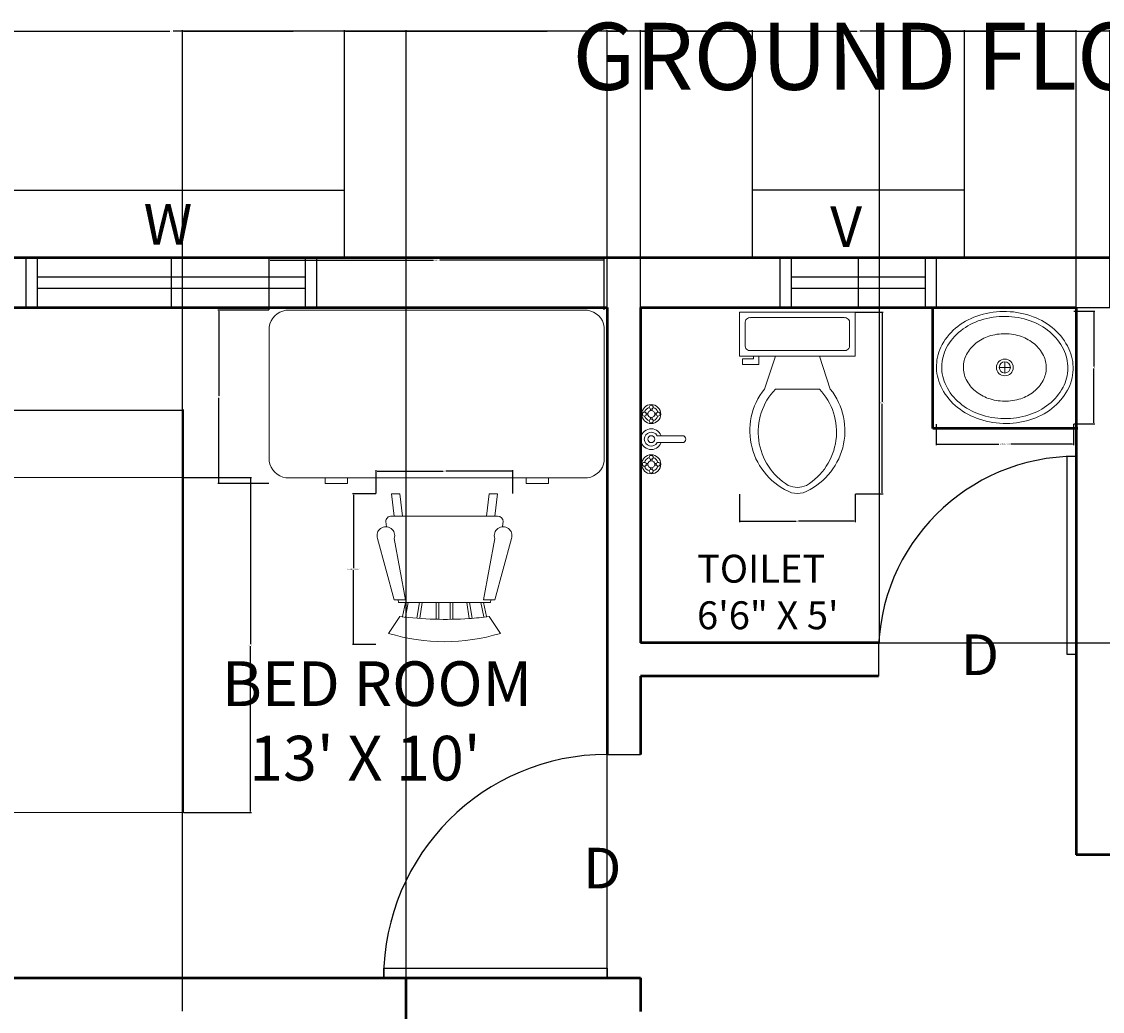
# Model space of a CAD drawing. Units: inches. Extents: x -73 to 1162, y -188 to 590.
# Tile 3 of 9: x 28 to 222, y 17 to 194. Entities that reach past the tile are written whole.
import ezdxf

# ---------------------------------------------------------------- set-up
doc = ezdxf.new("R2010")
doc.units = ezdxf.units.IN
doc.header["$MEASUREMENT"] = 0
for name, color, linetype, lineweight in [('A-ANNO-DIMS', 2, 'Continuous', 18), ('A-ANNO-TEXT', 7, 'Continuous', 25), ('A-AREA-IDEN', 2, 'Continuous', 25), ('A-DOOR', 3, 'Continuous', 25), ('A-FLOR-FIXT', 8, 'Continuous', 18), ('A-FURN', 8, 'Continuous', 18), ('A-GLAZ', 4, 'Continuous', 25), ('A-WALL', 7, 'Continuous', 50)]:
    doc.layers.add(name, color=color, linetype=linetype, lineweight=lineweight)
doc.styles.get("Standard").update_dxf_attribs({"font": 'arial.ttf'})
doc.dimstyles.get("Standard").update_dxf_attribs({"dimtxt": 0.18, "dimasz": 0.18, "dimexe": 0.18, "dimexo": 0.0625, "dimgap": 0.09, "dimtad": 0, "dimtih": 1, "dimtoh": 1, "dimdec": 1, "dimzin": 0, "dimdsep": 46, "dimlunit": 4, "dimtxsty": 'Standard', "dimcen": 0.09, "dimadec": 0, "dimazin": 0, "dimtfac": 1, "dimtdec": 1, "dimtofl": 0, "dimtmove": 0, "dimatfit": 3, "dimfxl": 1, "dimtolj": 1, "dimtzin": 0, "dimarcsym": 0})

# ---------------------------------------------------------------- blocks, each defined once
blk = doc.blocks.new('*U2')
for p, q in [((0, 0), (0, -6)), ((40, 0), (40, -6))]:
    blk.add_line(p, q)
blk.add_lwpolyline([(0, 0), (0, 40), (1.75, 40), (1.75, 0)], close=True)
blk.add_arc((0, 0), 40, 0, 90)
blk = doc.blocks.new('*U5')
for p, q in [((0, 0), (0, -100)), ((-900, 0), (-900, -100))]:
    blk.add_line(p, q)
blk.add_lwpolyline([(0, 0), (0, 900), (-43.75, 900), (-43.75, 0)], close=True)
blk.add_arc((0, 0), 900, 90, 180)
blk = doc.blocks.new('Bed - Queen')
for p, q in [((0, -80.00003), (0, 0)), ((0, 0), (59.99999, 0)), ((59.99999, 0), (59.99999, -80.00003)), ((7.99999, -1.2), (28.79998, -1.2)), ((7.99999, -14.4), (7.99999, -1.2)), ((28.79998, -1.2), (28.79998, -14.4)), ((31.19999, -1.2), (51.99999, -1.2)), ((31.19999, -14.4), (31.19999, -1.2)), ((51.99999, -1.2), (51.99999, -16.4)), ((0, -14.4), (44.8, -14.4)), ((59.99999, -29.6), (44.8, -14.4)), ((44.8, -14.4), (44.8, -29.6)), ((44.8, -16.8), (0, -16.8)), ((51.99999, -16.4), (46.79936, -16.4)), ((44.8, -29.6), (59.99999, -29.6)), ((59.99999, -80.00003), (0, -80.00003))]:
    blk.add_line(p, q)
blk = doc.blocks.new('Desk - 30 x 60 in.')
for p, q in [((-26.999995, 0), (26.999995, 0)), ((-29.999995, -27), (-29.999995, -3)), ((29.999995, -3), (29.999995, -27)), ((26.999995, -30), (-26.999995, -30)), ((-20.000005, -30), (-20.000005, -31)), ((-16.000005, -31), (-16.000005, -30)), ((15.999995, -31), (15.999995, -30)), ((19.999995, -30), (19.999995, -31)), ((-20.000005, -31), (-16.000005, -31)), ((19.999995, -31), (15.999995, -31))]:
    blk.add_line(p, q)
for centre, start, end in [((-26.499995, -3.5), 98.1301, 171.8699), ((26.499995, -3.5), 8.130102, 81.8699), ((-26.499995, -26.5), 188.1301, 261.8699), ((26.499995, -26.5), 278.1301, 351.8699)]:
    blk.add_arc(centre, 3.535534, start, end)
blk = doc.blocks.new('Chair - Rocking')
for p, q in [((-8, -4.5), (-10, -1.5)), ((8, -4.5), (10, -1.5)), ((-7.5, -4.5), (-7, -7)), ((-6.5, -7), (-7.02225, -4.43)), ((-4.5, -7), (-4.96674, -4.19951)), ((-4, -7), (-4.40532, -4.16272)), ((-1.5, -4.05012), (-1.5, -7)), ((-1, -7), (-1, -4.05012)), ((1, -7), (1, -4.04655)), ((1.5, -4.05012), (1.5, -7)), ((4, -7), (4.40187, -4.18694)), ((4.5, -7), (4.96761, -4.19437)), ((6.5, -7), (7, -4.4057)), ((7.5, -4.5), (7, -7)), ((-9, -7.5), (-12, -18.49999)), ((-7, -7.5), (-9, -7.5)), ((-9, -18.49999), (-7, -7.5)), ((-8.23428, -6.99939), (-8.3093, -7.47958)), ((-8.23041, -7), (8.23915, -7)), ((7, -7.5), (9, -7.5)), ((9, -18.49999), (7, -7.5)), ((8.31071, -7.48854), (8.23449, -7.00073)), ((9, -7.5), (12, -18.49999)), ((-10.36644, -20.64523), (-10.5, -21.49999)), ((10.5, -21.49999), (10.3575, -20.58798)), ((-9, -22.49999), (-9.5, -26.49999)), ((0, -22.49999), (-9.5, -22.49999)), ((-8, -26.49999), (-7.5, -22.49999)), ((0, -22.49999), (9.5, -22.49999)), ((8, -26.49999), (7.5, -22.49999)), ((9, -22.49999), (9.5, -26.49999)), ((-9.5, -26.49999), (-8, -26.49999)), ((9.5, -26.49999), (8, -26.49999))]:
    blk.add_line(p, q)
for centre, radius, start, end in [((0, -34.08333), 34.08333, 72.93847, 107.0615), ((0, -68.25004), 64.25, 93.92211, 97.15267), ((0, -68.25004), 64.25, 82.84733, 93.92211), ((-10.5, -18.99999), 1.58114, 161.5651, 18.43495), ((10.5, -18.99999), 1.58114, 161.5651, 18.43495), ((-9.5, -21.49999), 1, 180, 270), ((9.5, -21.49999), 1, 270, 0)]:
    blk.add_arc(centre, radius, start, end)
blk = doc.blocks.new('Sink - Oval top')
for p, q in [((-1, 0), (1, 0)), ((0, 1), (0, -1))]:
    blk.add_line(p, q)
for points in [[(-12.23, 0.39, 0.117634), (-11.46, -3.36, 0.104469), (-8.88, -6.8, 0.090016), (-5.08, -9.07, 0.08192), (-0.32, -10.02, 0.08192), (4.49, -9.38, 0.090016), (8.42, -7.36, 0.104469), (11.22, -4.09, 0.117634), (12.23, -0.39, 0.117634), (11.46, 3.36, 0.104469), (8.88, 6.8, 0.090016), (5.08, 9.07, 0.08192), (0.32, 10.02, 0.08192), (-4.49, 9.38, 0.090016), (-8.42, 7.36, 0.104469), (-11.22, 4.09, 0.117634)], [(-11.29, 0.16, 0.118622), (-10.52, -3.25, 0.104678), (-8.07, -6.36, 0.089562), (-4.54, -8.37, 0.081185), (-0.13, -9.15, 0.081185), (4.3, -8.49, 0.089562), (7.89, -6.58, 0.104678), (10.42, -3.55, 0.118622), (11.29, -0.16, 0.118622), (10.52, 3.25, 0.104678), (8.07, 6.36, 0.089562), (4.54, 8.37, 0.081185), (0.13, 9.15, 0.081185), (-4.3, 8.49, 0.089562), (-7.89, 6.58, 0.104678), (-10.42, 3.55, 0.118622)], [(-7.42, 0.08, 0.118283), (-6.91, -2.17, 0.104607), (-5.29, -4.21, 0.089718), (-2.97, -5.53, 0.081436), (-0.07, -6.04, 0.081436), (2.84, -5.59, 0.089718), (5.2, -4.33, 0.104607), (6.86, -2.32, 0.118283), (7.42, -0.08, 0.118283), (6.91, 2.17, 0.104607), (5.29, 4.21, 0.089718), (2.97, 5.53, 0.081436), (0.07, 6.04, 0.081436), (-2.84, 5.59, 0.089718), (-5.2, 4.33, 0.104607), (-6.86, 2.32, 0.118283)]]:
    blk.add_lwpolyline(points, format="xyb", close=True)
for radius in [1.5, 1]:
    blk.add_circle((0, 0), radius)
blk = doc.blocks.new('Toilet - top')
for p, q in [((9.5, -6), (9.5, -2)), ((-10, -8.5), (-8, -8.5)), ((-10, -9.5), (-10, -8.5)), ((-7, -9.5), (-10, -9.5)), ((-8, -8.5), (-8, -8)), ((-7, -8), (-7, -9.5)), ((-4, -8), (-6, -14)), ((4, -8), (6, -14)), ((4, -14), (-4, -14))]:
    blk.add_line(p, q)
blk.add_lwpolyline([(10.5, -8), (10.5, 0), (-10.5, 0), (-10.5, -8)], close=True)
for points in [[(8.5, -1), (-8.5, -1)], [(-9.5, -2), (-9.5, -6)], [(-8.5, -7), (8.5, -7)]]:
    blk.add_lwpolyline(points)
for centre, radius, start, end in [((-8.62, -1.88), 0.884, 81.8699, 188.1301), ((8.62, -1.88), 0.884, 351.8699, 98.1301), ((-8.62, -6.12), 0.884, 171.8699, 278.1301), ((8.62, -6.12), 0.884, 261.8699, 8.1301), ((3.52, -21.58), 12.17, 141.4691, 247.9714), ((4.2, -21.82), 11.33, 136.3677, 238.9468), ((-3.52, -21.58), 12.17, 292.0284, 38.5307), ((-4.2, -21.82), 11.33, 301.053, 43.6321), ((0, -27.88), 4, 245.7318, 294.2682), ((0, -29), 4, 254.8605, 285.1395)]:
    blk.add_arc(centre, radius, start, end)
blk = doc.blocks.new('Faucet - Bathroom top')
for p, q in [((-4.107, 0.125), (-4.375, 0.125)), ((-3.75, 0.4788), (-3.75, 0.75)), ((-3.5, 0.482), (-3.5, 0.75)), ((-3.1461, 0.125), (-2.875, 0.125)), ((3.143, 0.125), (2.875, 0.125)), ((3.5, 0.4788), (3.5, 0.75)), ((3.75, 0.482), (3.75, 0.75)), ((4.1039, 0.125), (4.375, 0.125)), ((-4.1039, -0.125), (-4.375, -0.125)), ((-3.75, -0.4821), (-3.75, -0.75)), ((-3.5, -0.4789), (-3.5, -0.75)), ((-3.143, -0.125), (-2.875, -0.125)), ((-0.5, -0.8639), (-0.5, -4.5)), ((0.5, -4.5), (0.5, -0.8631)), ((3.1461, -0.125), (2.875, -0.125)), ((3.5, -0.4821), (3.5, -0.75)), ((3.75, -0.4789), (3.75, -0.75)), ((4.107, -0.125), (4.375, -0.125))]:
    blk.add_line(p, q)
for centre, radius in [((-3.625, 0), 1.375), ((-4.625, 0), 0.2795), ((-3.625, 0), 0.5), ((-3.625, 1), 0.2795), ((-2.625, 0), 0.2795), ((0, 0), 0.5), ((3.625, 0), 1.375), ((2.625, 0), 0.2795), ((3.625, 0), 0.5), ((3.625, 1), 0.2795), ((4.625, 0), 0.2795), ((-3.625, -1), 0.2795), ((3.625, -1), 0.2795)]:
    blk.add_circle(centre, radius)
for centre, radius, start, end in [((-3.625, 0), 1, 105.2407, 164.2093), ((-3.625, 0), 1, 16.44125, 74.07887), ((0, 0), 1.5, 289.6514, 250.3603), ((0, 0), 1, 300.3431, 239.7554), ((3.625, 0), 1, 106.12, 164.0884), ((3.625, 0), 1, 16.23422, 73.90469), ((-3.625, 0), 1, 196.2342, 253.9047), ((-3.625, 0), 1, 286.12, 344.0884), ((3.625, 0), 1, 196.4413, 254.0789), ((3.625, 0), 1, 285.2407, 344.2093), ((0, -4.5), 0.5, 180, 0)]:
    blk.add_arc(centre, radius, start, end)
blk = doc.blocks.new('WIN-W')
for p, q in [((9, 57), (9, 62)), ((9, 62), (21, 62)), ((21, 62), (21, 0)), ((0, 57), (9, 57)), ((0, 5), (9, 5)), ((9, 5), (9, 0)), ((9, 0), (21, 0))]:
    blk.add_line(p, q)
blk = doc.blocks.new('VENT-V')
for p, q in [((0, 9), (0, 21)), ((38, 21), (0, 21)), ((38, 9), (38, 21)), ((5, 9), (0, 9)), ((5, 0), (5, 9)), ((33, 0), (33, 9)), ((33, 9), (38, 9))]:
    blk.add_line(p, q)
blk = doc.blocks.new('*D34')
at = {"layer": 'A-ANNO-DIMS', "color": 0, "lineweight": -2, "transparency": 16777216}
for p, q in [((-22.68, 112.85), (-22.68, 124.96)), ((-22.5, 124.78), (16.02, 124.78)), ((57.14, 124.78), (18.63, 124.78)), ((57.32, 112.85), (57.32, 124.96))]:
    blk.add_line(p, q, dxfattribs=at)
at = {"layer": 'A-ANNO-DIMS', "color": 0, "transparency": 16777216}
for points in [[(-22.5, 124.81), (-22.5, 124.75), (-22.68, 124.78)], [(57.14, 124.81), (57.14, 124.75), (57.32, 124.78)]]:
    blk.add_solid(points, dxfattribs=at)
at = {"layer": 'Defpoints', "color": 0, "transparency": 16777216}
for p in [(-22.68, 124.78), (-22.68, 112.78), (57.32, 112.78)]:
    blk.add_point(p, dxfattribs=at)
at = {"layer": 'A-ANNO-DIMS', "color": 0, "transparency": 16777216, "insert": (17.32, 124.78), "char_height": 0.18, "attachment_point": 5}
blk.add_mtext('\\A1;QUEEN BED 80 TYP.', dxfattribs=at)
blk = doc.blocks.new('*D35')
at = {"layer": 'A-ANNO-DIMS', "color": 0, "lineweight": -2, "transparency": 16777216}
for p, q in [((57.39, 112.78), (69.5, 112.78)), ((69.32, 112.6), (69.32, 82.97)), ((69.32, 52.96), (69.32, 82.6)), ((57.39, 52.78), (69.5, 52.78))]:
    blk.add_line(p, q, dxfattribs=at)
at = {"layer": 'A-ANNO-DIMS', "color": 0, "transparency": 16777216}
for points in [[(69.29, 112.6), (69.35, 112.6), (69.32, 112.78)], [(69.29, 52.96), (69.35, 52.96), (69.32, 52.78)]]:
    blk.add_solid(points, dxfattribs=at)
at = {"layer": 'Defpoints', "color": 0, "transparency": 16777216}
for p in [(57.32, 112.78), (69.32, 112.78), (57.32, 52.78)]:
    blk.add_point(p, dxfattribs=at)
at = {"layer": 'A-ANNO-DIMS', "color": 0, "transparency": 16777216, "insert": (69.32, 82.78), "char_height": 0.18, "attachment_point": 5}
blk.add_mtext('\\A1;60 TYP.', dxfattribs=at)
blk = doc.blocks.new('*D42')
at = {"layer": 'A-ANNO-DIMS', "color": 0, "lineweight": -2, "transparency": 16777216}
for p, q in [((72.66, 142.77), (72.66, 151.88)), ((72.84, 151.7), (102.07, 151.7)), ((132.48, 151.7), (103.25, 151.7)), ((132.66, 142.77), (132.66, 151.88))]:
    blk.add_line(p, q, dxfattribs=at)
at = {"layer": 'A-ANNO-DIMS', "color": 0, "transparency": 16777216}
for points in [[(72.84, 151.73), (72.84, 151.67), (72.66, 151.7)], [(132.48, 151.73), (132.48, 151.67), (132.66, 151.7)]]:
    blk.add_solid(points, dxfattribs=at)
at = {"layer": 'Defpoints', "color": 0, "transparency": 16777216}
for p in [(132.66, 151.7), (72.66, 142.7), (132.66, 142.7)]:
    blk.add_point(p, dxfattribs=at)
at = {"layer": 'A-ANNO-DIMS', "color": 0, "transparency": 16777216, "insert": (102.66, 151.7), "char_height": 0.18, "attachment_point": 5}
blk.add_mtext('\\A1;DESK 60', dxfattribs=at)
blk = doc.blocks.new('*D43')
at = {"layer": 'A-ANNO-DIMS', "color": 0, "lineweight": -2, "transparency": 16777216}
for p, q in [((72.6, 142.7), (63.48, 142.7)), ((63.66, 142.52), (63.66, 127.39)), ((63.66, 111.88), (63.66, 127.02)), ((72.6, 111.7), (63.48, 111.7))]:
    blk.add_line(p, q, dxfattribs=at)
at = {"layer": 'A-ANNO-DIMS', "color": 0, "transparency": 16777216}
for points in [[(63.63, 142.52), (63.69, 142.52), (63.66, 142.7)], [(63.63, 111.88), (63.69, 111.88), (63.66, 111.7)]]:
    blk.add_solid(points, dxfattribs=at)
at = {"layer": 'Defpoints', "color": 0, "transparency": 16777216}
for p in [(63.66, 142.7), (72.66, 142.7), (72.66, 111.7)]:
    blk.add_point(p, dxfattribs=at)
at = {"layer": 'A-ANNO-DIMS', "color": 0, "transparency": 16777216, "insert": (63.66, 127.2), "char_height": 0.18, "attachment_point": 5}
blk.add_mtext('\\A1;31', dxfattribs=at)
blk = doc.blocks.new('*D44')
at = {"layer": 'A-ANNO-DIMS', "color": 0, "lineweight": -2, "transparency": 16777216}
for p, q in [((91.78, 109.87), (87.61, 109.87)), ((87.79, 109.69), (87.79, 96.55)), ((87.79, 83.05), (87.79, 96.18)), ((91.78, 82.87), (87.61, 82.87))]:
    blk.add_line(p, q, dxfattribs=at)
at = {"layer": 'A-ANNO-DIMS', "color": 0, "transparency": 16777216}
for points in [[(87.76, 109.69), (87.82, 109.69), (87.79, 109.87)], [(87.76, 83.05), (87.82, 83.05), (87.79, 82.87)]]:
    blk.add_solid(points, dxfattribs=at)
at = {"layer": 'Defpoints', "color": 0, "transparency": 16777216}
for p in [(91.84, 109.87), (87.79, 82.87), (91.84, 82.87)]:
    blk.add_point(p, dxfattribs=at)
at = {"layer": 'A-ANNO-DIMS', "color": 0, "transparency": 16777216, "insert": (87.79, 96.37), "char_height": 0.18, "attachment_point": 5}
blk.add_mtext('\\A1;ROCKING CHAIR 27', dxfattribs=at)
blk = doc.blocks.new('*D45')
at = {"layer": 'A-ANNO-DIMS', "color": 0, "lineweight": -2, "transparency": 16777216}
for p, q in [((91.84, 109.93), (91.84, 114.1)), ((92.02, 113.92), (103.84, 113.92)), ((116.09, 113.92), (104.28, 113.92)), ((116.27, 109.93), (116.27, 114.1))]:
    blk.add_line(p, q, dxfattribs=at)
at = {"layer": 'A-ANNO-DIMS', "color": 0, "transparency": 16777216}
for points in [[(92.02, 113.95), (92.02, 113.89), (91.84, 113.92)], [(116.09, 113.95), (116.09, 113.89), (116.27, 113.92)]]:
    blk.add_solid(points, dxfattribs=at)
at = {"layer": 'Defpoints', "color": 0, "transparency": 16777216}
for p in [(91.84, 113.92), (91.84, 109.87), (116.27, 109.87)]:
    blk.add_point(p, dxfattribs=at)
at = {"layer": 'A-ANNO-DIMS', "color": 0, "transparency": 16777216, "insert": (104.06, 113.92), "char_height": 0.18, "attachment_point": 5}
blk.add_mtext('\\A1;24', dxfattribs=at)
blk = doc.blocks.new('*D54')
at = {"layer": 'A-ANNO-DIMS', "color": 0, "lineweight": -2, "transparency": 16777216}
for p, q in [((192.1, 122.34), (192.1, 118.54)), ((216.65, 122.34), (216.65, 118.54)), ((192.28, 118.72), (203.32, 118.72)), ((216.47, 118.72), (205.42, 118.72))]:
    blk.add_line(p, q, dxfattribs=at)
at = {"layer": 'A-ANNO-DIMS', "color": 0, "transparency": 16777216}
for points in [[(192.28, 118.75), (192.28, 118.69), (192.1, 118.72)], [(216.47, 118.75), (216.47, 118.69), (216.65, 118.72)]]:
    blk.add_solid(points, dxfattribs=at)
at = {"layer": 'Defpoints', "color": 0, "transparency": 16777216}
for p in [(192.1, 122.4), (216.65, 122.4), (216.65, 118.72)]:
    blk.add_point(p, dxfattribs=at)
at = {"layer": 'A-ANNO-DIMS', "color": 0, "transparency": 16777216, "insert": (204.37, 118.72), "char_height": 0.18, "attachment_point": 5}
blk.add_mtext('\\A1;WASH BASIN 25', dxfattribs=at)
blk = doc.blocks.new('*D55')
at = {"layer": 'A-ANNO-DIMS', "color": 0, "lineweight": -2, "transparency": 16777216}
for p, q in [((216.71, 142.54), (220.51, 142.54)), ((220.33, 142.36), (220.33, 132.65)), ((220.33, 122.58), (220.33, 132.29)), ((216.71, 122.4), (220.51, 122.4))]:
    blk.add_line(p, q, dxfattribs=at)
at = {"layer": 'A-ANNO-DIMS', "color": 0, "transparency": 16777216}
for points in [[(220.3, 142.36), (220.36, 142.36), (220.33, 142.54)], [(220.3, 122.58), (220.36, 122.58), (220.33, 122.4)]]:
    blk.add_solid(points, dxfattribs=at)
at = {"layer": 'Defpoints', "color": 0, "transparency": 16777216}
for p in [(216.65, 142.54), (220.33, 142.54), (216.65, 122.4)]:
    blk.add_point(p, dxfattribs=at)
at = {"layer": 'A-ANNO-DIMS', "color": 0, "transparency": 16777216, "insert": (220.33, 132.47), "char_height": 0.18, "attachment_point": 5}
blk.add_mtext('\\A1;20', dxfattribs=at)
blk = doc.blocks.new('*D56')
at = {"layer": 'A-ANNO-DIMS', "color": 0, "lineweight": -2, "transparency": 16777216}
for p, q in [((177.62, 142.37), (182.62, 142.37)), ((182.44, 142.19), (182.44, 126.3)), ((182.44, 110.04), (182.44, 125.93)), ((177.62, 109.86), (182.62, 109.86))]:
    blk.add_line(p, q, dxfattribs=at)
at = {"layer": 'A-ANNO-DIMS', "color": 0, "transparency": 16777216}
for points in [[(182.41, 142.19), (182.47, 142.19), (182.44, 142.37)], [(182.41, 110.04), (182.47, 110.04), (182.44, 109.86)]]:
    blk.add_solid(points, dxfattribs=at)
at = {"layer": 'Defpoints', "color": 0, "transparency": 16777216}
for p in [(177.56, 142.37), (182.44, 142.37), (177.56, 109.86)]:
    blk.add_point(p, dxfattribs=at)
at = {"layer": 'A-ANNO-DIMS', "color": 0, "transparency": 16777216, "insert": (182.44, 126.11), "char_height": 0.18, "attachment_point": 5}
blk.add_mtext('\\A1;WC 33', dxfattribs=at)
blk = doc.blocks.new('*D57')
at = {"layer": 'A-ANNO-DIMS', "color": 0, "lineweight": -2, "transparency": 16777216}
for p, q in [((156.9, 109.8), (156.9, 104.8)), ((177.56, 109.8), (177.56, 104.8)), ((157.08, 104.98), (167.03, 104.98)), ((177.38, 104.98), (167.43, 104.98))]:
    blk.add_line(p, q, dxfattribs=at)
at = {"layer": 'A-ANNO-DIMS', "color": 0, "transparency": 16777216}
for points in [[(157.08, 105.01), (157.08, 104.95), (156.9, 104.98)], [(177.38, 105.01), (177.38, 104.95), (177.56, 104.98)]]:
    blk.add_solid(points, dxfattribs=at)
at = {"layer": 'Defpoints', "color": 0, "transparency": 16777216}
for p in [(156.9, 109.86), (177.56, 109.86), (177.56, 104.98)]:
    blk.add_point(p, dxfattribs=at)
at = {"layer": 'A-ANNO-DIMS', "color": 0, "transparency": 16777216, "insert": (167.23, 104.98), "char_height": 0.18, "attachment_point": 5}
blk.add_mtext('\\A1;21', dxfattribs=at)
blk = doc.blocks.new('*D60')
at = {"layer": 'A-ANNO-DIMS', "color": 0, "lineweight": -2, "transparency": 16777216}
for p, q in [((86.17, 164.25), (86.17, 192.86)), ((86.35, 192.68), (122.45, 192.68)), ((158.99, 192.68), (122.89, 192.68)), ((159.17, 164.25), (159.17, 192.86))]:
    blk.add_line(p, q, dxfattribs=at)
at = {"layer": 'A-ANNO-DIMS', "color": 0, "transparency": 16777216}
for points in [[(86.35, 192.71), (86.35, 192.65), (86.17, 192.68)], [(158.99, 192.71), (158.99, 192.65), (159.17, 192.68)]]:
    blk.add_solid(points, dxfattribs=at)
at = {"layer": 'Defpoints', "color": 0, "transparency": 16777216}
for p in [(159.17, 192.68), (86.17, 164.18), (159.17, 164.18)]:
    blk.add_point(p, dxfattribs=at)
at = {"layer": 'A-ANNO-DIMS', "color": 0, "transparency": 16777216, "insert": (122.67, 192.68), "char_height": 0.18, "attachment_point": 5}
blk.add_mtext('\\A1;73', dxfattribs=at)
blk = doc.blocks.new('*D61')
at = {"layer": 'A-ANNO-DIMS', "color": 0, "lineweight": -2, "transparency": 16777216}
for p, q in [((197.17, 164.25), (197.17, 192.86)), ((197.35, 192.68), (219.95, 192.68)), ((242.99, 192.68), (220.39, 192.68)), ((243.17, 164.25), (243.17, 192.86))]:
    blk.add_line(p, q, dxfattribs=at)
at = {"layer": 'A-ANNO-DIMS', "color": 0, "transparency": 16777216}
for points in [[(197.35, 192.71), (197.35, 192.65), (197.17, 192.68)], [(242.99, 192.71), (242.99, 192.65), (243.17, 192.68)]]:
    blk.add_solid(points, dxfattribs=at)
at = {"layer": 'Defpoints', "color": 0, "transparency": 16777216}
for p in [(243.17, 192.68), (197.17, 164.18), (243.17, 164.18)]:
    blk.add_point(p, dxfattribs=at)
at = {"layer": 'A-ANNO-DIMS', "color": 0, "transparency": 16777216, "insert": (220.17, 192.68), "char_height": 0.18, "attachment_point": 5}
blk.add_mtext('\\A1;46', dxfattribs=at)
blk = doc.blocks.new('*D87')
at = {"layer": 'A-ANNO-DIMS', "color": 0, "lineweight": -2, "transparency": 16777216}
for p, q in [((133.17, 143.25), (133.17, 192.86)), ((133.35, 192.68), (136.02, 192.68)), ((138.99, 192.68), (136.32, 192.68)), ((139.17, 143.25), (139.17, 192.86))]:
    blk.add_line(p, q, dxfattribs=at)
at = {"layer": 'A-ANNO-DIMS', "color": 0, "transparency": 16777216}
for points in [[(133.35, 192.71), (133.35, 192.65), (133.17, 192.68)], [(138.99, 192.71), (138.99, 192.65), (139.17, 192.68)]]:
    blk.add_solid(points, dxfattribs=at)
at = {"layer": 'Defpoints', "color": 0, "transparency": 16777216}
for p in [(139.17, 192.68), (133.17, 143.18), (139.17, 143.18)]:
    blk.add_point(p, dxfattribs=at)
at = {"layer": 'A-ANNO-DIMS', "color": 0, "transparency": 16777216, "insert": (136.17, 192.68), "char_height": 0.18, "attachment_point": 5}
blk.add_mtext('\\A1;6', dxfattribs=at)
blk = doc.blocks.new('*D88')
at = {"layer": 'A-ANNO-DIMS', "color": 0, "lineweight": -2, "transparency": 16777216}
for p, q in [((-22.83, 143.25), (-22.83, 192.86)), ((-22.65, 192.68), (54.89, 192.68)), ((132.99, 192.68), (55.45, 192.68)), ((133.17, 143.25), (133.17, 192.86))]:
    blk.add_line(p, q, dxfattribs=at)
at = {"layer": 'A-ANNO-DIMS', "color": 0, "transparency": 16777216}
for points in [[(-22.65, 192.71), (-22.65, 192.65), (-22.83, 192.68)], [(132.99, 192.71), (132.99, 192.65), (133.17, 192.68)]]:
    blk.add_solid(points, dxfattribs=at)
at = {"layer": 'Defpoints', "color": 0, "transparency": 16777216}
for p in [(133.17, 192.68), (-22.83, 143.18), (133.17, 143.18)]:
    blk.add_point(p, dxfattribs=at)
at = {"layer": 'A-ANNO-DIMS', "color": 0, "transparency": 16777216, "insert": (55.17, 192.68), "char_height": 0.18, "attachment_point": 5}
blk.add_mtext('\\A1;156', dxfattribs=at)
blk = doc.blocks.new('*D89')
at = {"layer": 'A-ANNO-DIMS', "color": 0, "lineweight": -2, "transparency": 16777216}
for p, q in [((139.17, 143.25), (139.17, 192.86)), ((139.35, 192.68), (177.95, 192.68)), ((216.99, 192.68), (178.39, 192.68)), ((217.17, 143.25), (217.17, 192.86))]:
    blk.add_line(p, q, dxfattribs=at)
at = {"layer": 'A-ANNO-DIMS', "color": 0, "transparency": 16777216}
for points in [[(139.35, 192.71), (139.35, 192.65), (139.17, 192.68)], [(216.99, 192.71), (216.99, 192.65), (217.17, 192.68)]]:
    blk.add_solid(points, dxfattribs=at)
at = {"layer": 'Defpoints', "color": 0, "transparency": 16777216}
for p in [(217.17, 192.68), (139.17, 143.18), (217.17, 143.18)]:
    blk.add_point(p, dxfattribs=at)
at = {"layer": 'A-ANNO-DIMS', "color": 0, "transparency": 16777216, "insert": (178.17, 192.68), "char_height": 0.18, "attachment_point": 5}
blk.add_mtext('\\A1;78', dxfattribs=at)
blk = doc.blocks.new('*D90')
at = {"layer": 'A-ANNO-DIMS', "color": 0, "lineweight": -2, "transparency": 16777216}
for p, q in [((217.17, 143.25), (217.17, 192.86)), ((217.35, 192.68), (220.02, 192.68)), ((222.99, 192.68), (220.32, 192.68)), ((223.17, 143.25), (223.17, 192.86))]:
    blk.add_line(p, q, dxfattribs=at)
at = {"layer": 'A-ANNO-DIMS', "color": 0, "transparency": 16777216}
for points in [[(217.35, 192.71), (217.35, 192.65), (217.17, 192.68)], [(222.99, 192.71), (222.99, 192.65), (223.17, 192.68)]]:
    blk.add_solid(points, dxfattribs=at)
at = {"layer": 'Defpoints', "color": 0, "transparency": 16777216}
for p in [(223.17, 192.68), (217.17, 143.18), (223.17, 143.18)]:
    blk.add_point(p, dxfattribs=at)
at = {"layer": 'A-ANNO-DIMS', "color": 0, "transparency": 16777216, "insert": (220.17, 192.68), "char_height": 0.18, "attachment_point": 5}
blk.add_mtext('\\A1;6', dxfattribs=at)
blk = doc.blocks.new('*D93')
at = {"layer": 'A-ANNO-DIMS', "color": 0, "lineweight": -2, "transparency": 16777216}
for p, q in [((139.23, 143.18), (541.85, 143.18)), ((541.67, 143), (541.67, 113.37)), ((541.67, 83.36), (541.67, 113)), ((139.23, 83.18), (541.85, 83.18))]:
    blk.add_line(p, q, dxfattribs=at)
at = {"layer": 'A-ANNO-DIMS', "color": 0, "transparency": 16777216}
for points in [[(541.64, 143), (541.7, 143), (541.67, 143.18)], [(541.64, 83.36), (541.7, 83.36), (541.67, 83.18)]]:
    blk.add_solid(points, dxfattribs=at)
at = {"layer": 'Defpoints', "color": 0, "transparency": 16777216}
for p in [(139.17, 143.18), (139.17, 83.18), (541.67, 83.18)]:
    blk.add_point(p, dxfattribs=at)
at = {"layer": 'A-ANNO-DIMS', "color": 0, "transparency": 16777216, "insert": (541.67, 113.18), "char_height": 0.18, "attachment_point": 5}
blk.add_mtext('\\A1;60', dxfattribs=at)
blk = doc.blocks.new('*D95')
at = {"layer": 'A-ANNO-DIMS', "color": 0, "lineweight": -2, "transparency": 16777216}
for p, q in [((97.17, 23.25), (97.17, 192.86)), ((97.35, 192.68), (114.95, 192.68)), ((132.99, 192.68), (115.39, 192.68)), ((133.17, 23.25), (133.17, 192.86))]:
    blk.add_line(p, q, dxfattribs=at)
at = {"layer": 'A-ANNO-DIMS', "color": 0, "transparency": 16777216}
for points in [[(97.35, 192.71), (97.35, 192.65), (97.17, 192.68)], [(132.99, 192.71), (132.99, 192.65), (133.17, 192.68)]]:
    blk.add_solid(points, dxfattribs=at)
at = {"layer": 'Defpoints', "color": 0, "transparency": 16777216}
for p in [(133.17, 192.68), (97.17, 23.18), (133.17, 23.18)]:
    blk.add_point(p, dxfattribs=at)
at = {"layer": 'A-ANNO-DIMS', "color": 0, "transparency": 16777216, "insert": (115.17, 192.68), "char_height": 0.18, "attachment_point": 5}
blk.add_mtext('\\A1;36', dxfattribs=at)
blk = doc.blocks.new('*D96')
at = {"layer": 'A-ANNO-DIMS', "color": 0, "lineweight": -2, "transparency": 16777216}
for p, q in [((181.91, 83.25), (181.91, 192.86)), ((182.09, 192.68), (199.08, 192.68)), ((216.99, 192.68), (200.01, 192.68)), ((217.17, 83.25), (217.17, 192.86))]:
    blk.add_line(p, q, dxfattribs=at)
at = {"layer": 'A-ANNO-DIMS', "color": 0, "transparency": 16777216}
for points in [[(182.09, 192.71), (182.09, 192.65), (181.91, 192.68)], [(216.99, 192.71), (216.99, 192.65), (217.17, 192.68)]]:
    blk.add_solid(points, dxfattribs=at)
at = {"layer": 'Defpoints', "color": 0, "transparency": 16777216}
for p in [(217.17, 192.68), (181.91, 83.18), (217.17, 83.18)]:
    blk.add_point(p, dxfattribs=at)
at = {"layer": 'A-ANNO-DIMS', "color": 0, "transparency": 16777216, "insert": (199.54, 192.68), "char_height": 0.18, "attachment_point": 5}
blk.add_mtext('\\A1;35.256', dxfattribs=at)
blk = doc.blocks.new('*D99')
at = {"layer": 'A-ANNO-DIMS', "color": 0, "lineweight": -2, "transparency": 16777216}
for p, q in [((57.17, 17.25), (57.17, 192.86)), ((57.35, 192.68), (76.95, 192.68)), ((96.99, 192.68), (77.39, 192.68)), ((97.17, 17.25), (97.17, 192.86))]:
    blk.add_line(p, q, dxfattribs=at)
at = {"layer": 'A-ANNO-DIMS', "color": 0, "transparency": 16777216}
for points in [[(57.35, 192.71), (57.35, 192.65), (57.17, 192.68)], [(96.99, 192.71), (96.99, 192.65), (97.17, 192.68)]]:
    blk.add_solid(points, dxfattribs=at)
at = {"layer": 'Defpoints', "color": 0, "transparency": 16777216}
for p in [(97.17, 192.68), (57.17, 17.18), (97.17, 17.18)]:
    blk.add_point(p, dxfattribs=at)
at = {"layer": 'A-ANNO-DIMS', "color": 0, "transparency": 16777216, "insert": (77.17, 192.68), "char_height": 0.18, "attachment_point": 5}
blk.add_mtext('\\A1;40', dxfattribs=at)

msp = doc.modelspace()

# ---------------------------------------------------------------- linework, layer by layer
at = {"layer": 'A-GLAZ'}
for p, q in [((31.17, 143.1844), (31.17, 152.1844)), ((55.17, 143.1844), (55.17, 152.1844)), ((79.17, 143.1844), (79.17, 152.1844)), ((166.17, 143.1844), (166.17, 152.1844)), ((178.17, 143.1844), (178.17, 152.1844)), ((190.17, 143.1844), (190.17, 152.1844)), ((31.17, 148.6844), (79.17, 148.6844)), ((166.17, 148.6844), (190.17, 148.6844)), ((31.17, 146.6844), (79.17, 146.6844)), ((166.17, 146.6844), (190.17, 146.6844))]:
    msp.add_line(p, q, dxfattribs=at)
at = {"layer": 'A-WALL'}
for p, q in [((-31.83, 152.1844), (139.17, 152.1844)), ((139.17, 152.1844), (223.17, 152.1844)), ((-22.83, 143.1844), (133.17, 143.1844)), ((133.17, 143.1844), (133.17, 63.1844)), ((139.17, 143.1844), (139.17, 83.1844)), ((139.17, 143.1844), (217.17, 143.1844)), ((191.5125, 121.5547), (191.5125, 143.1844)), ((217.17, 143.1844), (217.17, 83.1844)), ((217.4523, 121.5547), (191.5125, 121.5547)), ((181.9138, 83.1844), (139.17, 83.1844)), ((217.17, 83.1844), (217.17, 77.1844)), ((181.7369, 77.1844), (139.17, 77.1844)), ((139.17, 77.1844), (139.17, 63.1844)), ((217.17, 77.1844), (217.17, 45.1844)), ((223.17, 45.1844), (217.17, 45.1844)), ((-22.83, 23.1844), (139.17, 23.1844)), ((97.17, 15.4344), (97.17, 23.1844)), ((139.17, 23.1844), (139.17, 17.1844))]:
    msp.add_line(p, q, dxfattribs=at)

# ---------------------------------------------------------------- block references
at = {"layer": 'A-DOOR', "xscale": 0.0393700787401575, "yscale": 0.0393700787401575, "zscale": 0.0393700787401575}
msp.add_blockref('*U5', (217.17, 81.1215), dxfattribs=at)
at = {"layer": 'A-DOOR', "rotation": 90}
msp.add_blockref('*U2', (133.17, 23.1844), dxfattribs=at)
at = {"layer": 'A-FLOR-FIXT', "xscale": 0.9837798500981108, "yscale": 0.9837798500981108, "zscale": 0.9837798500981108}
msp.add_blockref('Toilet - top', (167.2302, 142.3691), dxfattribs=at)
at = {"layer": 'A-FLOR-FIXT'}
msp.add_blockref('Sink - Oval top', (204.3716, 132.4699), dxfattribs=at)
at = {"layer": 'A-FLOR-FIXT', "xscale": 1.239598083049878, "yscale": 1.239598083049878, "zscale": 1.239598083049878, "rotation": 90}
msp.add_blockref('Faucet - Bathroom top', (141.0716, 119.6307), dxfattribs=at)
at = {"layer": 'A-FURN'}
msp.add_blockref('Desk - 30 x 60 in.', (102.6623, 142.7039), dxfattribs=at)
for name, p, rotation in [('Bed - Queen', (-22.6767, 52.7839), 90), ('Chair - Rocking', (104.0555, 83.3678), 180)]:
    msp.add_blockref(name, p, dxfattribs=dict(at, rotation=rotation))
at = {"layer": 'A-GLAZ', "rotation": 89.99999999999999}
msp.add_blockref('WIN-W', (86.1704, 143.1844), dxfattribs=at)
at = {"layer": 'A-GLAZ'}
msp.add_blockref('VENT-V', (159.17, 143.184), dxfattribs=at)

# ---------------------------------------------------------------- texts
at = {"layer": 'A-ANNO-TEXT'}
for s, p in [('W', (50.1847, 154.461)), ('V', (173.1016, 154.0395)), ('D', (196.5079, 77.389)), ('D', (128.8796, 39.1954))]:
    msp.add_text(s, height=7.2829, dxfattribs=at).set_placement(p)
at = {"layer": 'A-ANNO-TEXT', "insert": (126.968, 194.1746), "char_height": 12, "attachment_point": 1}
msp.add_mtext_dynamic_manual_height_columns('GROUND FLOOR PLAN', width=198.609453, gutter_width=1, heights=[0], dxfattribs=at)
at = {"layer": 'A-AREA-IDEN', "attachment_point": 1}
for s, insert, char_height in [('TOILET\\P6\'6" X 5\'', (149.2675, 98.9372), 5), ("BED ROOM\\P  13' X 10'", (64.2065, 79.8553), 8)]:
    msp.add_mtext_dynamic_manual_height_columns(s, width=71.534965, gutter_width=1, heights=[0], dxfattribs=dict(at, insert=insert, char_height=char_height))

# ---------------------------------------------------------------- dimensions: what is measured, and where the dimension line sits
at = {"layer": 'A-ANNO-DIMS'}
for base, p1, p2, override, picture, middle in [((133.17, 192.6844), (-22.83, 143.1844), (133.17, 143.1844), {"dimdec": 0, "dimlfac": 1, "dimrnd": 0, "dimzin": 0, "dimdsep": 46, "dimlunit": 2}, '*D88', (55.17, 192.6844)), ((97.17, 192.6844), (57.17, 17.1844), (97.17, 17.1844), {"dimdec": 0, "dimlfac": 1, "dimrnd": 0, "dimzin": 0, "dimdsep": 46, "dimlunit": 2}, '*D99', (77.17, 192.6844)), ((159.17, 192.6844), (86.17, 164.1844), (159.17, 164.1844), {"dimdec": 0, "dimlfac": 1, "dimrnd": 0, "dimzin": 0, "dimdsep": 46, "dimlunit": 2}, '*D60', (122.67, 192.6844)), ((133.17, 192.6844), (97.17, 23.1844), (133.17, 23.1844), {"dimdec": 0, "dimlfac": 1, "dimrnd": 0, "dimzin": 0, "dimdsep": 46, "dimlunit": 2}, '*D95', (115.17, 192.6844)), ((139.17, 192.6844), (133.17, 143.1844), (139.17, 143.1844), {"dimdec": 0, "dimlfac": 1, "dimrnd": 0, "dimzin": 0, "dimdsep": 46, "dimlunit": 2}, '*D87', (136.17, 192.6844)), ((217.17, 192.6844), (139.17, 143.1844), (217.17, 143.1844), {"dimdec": 0, "dimlfac": 1, "dimrnd": 0, "dimzin": 0, "dimdsep": 46, "dimlunit": 2}, '*D89', (178.17, 192.6844)), ((217.17, 192.6844), (181.9138, 83.1844), (217.17, 83.1844), {"dimdec": 3, "dimlfac": 1, "dimrnd": 0, "dimzin": 0, "dimdsep": 46, "dimlunit": 2}, '*D96', (199.5419, 192.6844)), ((243.17, 192.6844), (197.17, 164.1844), (243.17, 164.1844), {"dimdec": 0, "dimlfac": 1, "dimrnd": 0, "dimzin": 0, "dimdsep": 46, "dimlunit": 2}, '*D61', (220.17, 192.6844)), ((223.17, 192.6844), (217.17, 143.1844), (223.17, 143.1844), {"dimdec": 0, "dimlfac": 1, "dimrnd": 0, "dimzin": 0, "dimdsep": 46, "dimlunit": 2}, '*D90', (220.17, 192.6844)), ((177.5599, 104.9823), (156.9005, 109.8588), (177.5599, 109.8588), {"dimdec": 0, "dimrnd": 0, "dimzin": 0, "dimlunit": 2}, '*D57', (167.2302, 104.9823))]:
    dim = msp.add_linear_dim(base=base, p1=p1, p2=p2, dimstyle='Standard', override=override, dxfattribs=at)
    dim.commit()
    dim.dimension.update_dxf_attribs({"geometry": picture, "text_midpoint": middle})
for base, p1, p2, text, picture, middle in [((132.6623, 151.7039), (72.6623, 142.7039), (132.6623, 142.7039), 'DESK <>', '*D42', (102.6623, 151.7039)), ((216.647, 118.719), (192.0961, 122.4016), (216.647, 122.4016), 'WASH BASIN <>', '*D54', (204.3716, 118.719))]:
    dim = msp.add_linear_dim(base=base, p1=p1, p2=p2, text=text, dimstyle='Standard', override={"dimdec": 0, "dimrnd": 0, "dimzin": 0, "dimlunit": 2}, dxfattribs=at)
    dim.commit()
    dim.dimension.update_dxf_attribs({"geometry": picture, "text_midpoint": middle})
for base, p1, p2, angle, override, picture, middle in [((63.6623, 142.7039), (72.6623, 111.7039), (72.6623, 142.7039), 90, {"dimdec": 0, "dimrnd": 0, "dimzin": 0, "dimlunit": 2}, '*D43', (63.6623, 127.2039)), ((541.67, 83.1844), (139.17, 143.1844), (139.17, 83.1844), 90, {"dimdec": 0, "dimlfac": 1, "dimrnd": 0, "dimzin": 0, "dimdsep": 46, "dimlunit": 2}, '*D93', (541.67, 113.1844)), ((220.3296, 142.5382), (216.647, 122.4016), (216.647, 142.5382), 90, {"dimdec": 0, "dimrnd": 0, "dimzin": 0, "dimlunit": 2}, '*D55', (220.3296, 132.4699)), ((91.8379, 113.9178), (116.273, 109.8678), (91.8379, 109.8678), 180, {"dimdec": 0, "dimrnd": 0, "dimzin": 0, "dimlunit": 2}, '*D45', (104.0555, 113.9178))]:
    dim = msp.add_linear_dim(base=base, p1=p1, p2=p2, angle=angle, dimstyle='Standard', override=override, dxfattribs=at)
    dim.commit()
    dim.dimension.update_dxf_attribs({"geometry": picture, "text_midpoint": middle})
for base, p1, p2, angle, text, picture, middle in [((182.4364, 142.3691), (177.5599, 109.8588), (177.5599, 142.3691), 90, 'WC <>', '*D56', (182.4364, 126.1139)), ((-22.6767, 124.7839), (57.3233, 112.7839), (-22.6767, 112.7839), 180, 'QUEEN BED <> TYP.', '*D34', (17.3233, 124.7839)), ((69.3233, 112.7839), (57.3233, 52.7839), (57.3233, 112.7839), 90, '<> TYP.', '*D35', (69.3233, 82.7839)), ((87.7879, 82.8678), (91.8379, 109.8678), (91.8379, 82.8678), 270, 'ROCKING CHAIR <>', '*D44', (87.7879, 96.3678))]:
    dim = msp.add_linear_dim(base=base, p1=p1, p2=p2, angle=angle, text=text, dimstyle='Standard', override={"dimdec": 0, "dimrnd": 0, "dimzin": 0, "dimlunit": 2}, dxfattribs=at)
    dim.commit()
    dim.dimension.update_dxf_attribs({"geometry": picture, "text_midpoint": middle})

doc.saveas('drawing.dxf')
